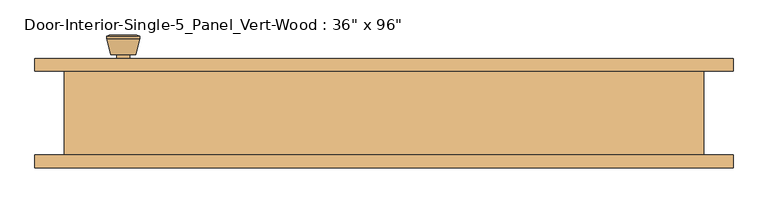
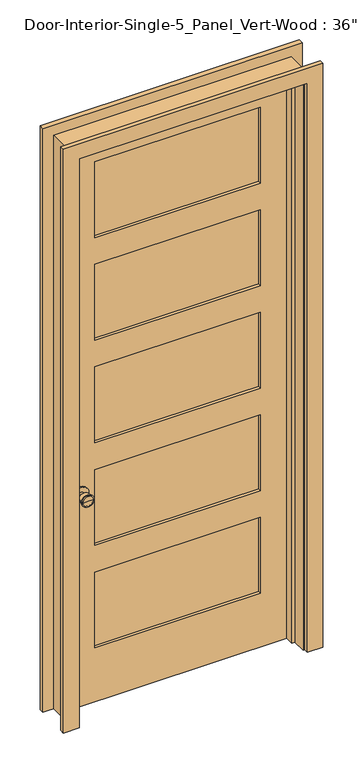
"""IFC4 building model written with IfcOpenShell, lengths in millimetres: door geometry."""

from ifc_helpers import new_model, si_unit, point, frame, frame_2d, origin, place, context, project, spatial, polyline, circle_curve, trimmed, segment, composite_curve, outline, extrude, faceted_brep, source, transform, mapped, element, save
from ifc_brep_helpers import plane_surface, cylinder_surface, revolved_surface, advanced_brep


def door_7b78131b(model_context):
    return source(origin(), model_context, "Body", "SolidModel", [
        advanced_brep(
        [(-393.7, 19.4, 914.4), (-383.7, 19.4, 914.4), (-403.7, 19.4, 914.4), (-373.2241324, -29.6, 914.4), (-393.7, -29.6, 914.4), (-414.1758676, -29.6, 914.4), (-368.7, -27.7721319, 914.4), (-418.7, -27.7721319, 914.4), (-368.7, -24.3084537, 914.4), (-418.7, -24.3084537, 914.4), (-375.063764, 0.4, 914.4), (-412.336236, 0.4, 914.4), (-383.7, 0.4, 914.4), (-403.7, 0.4, 914.4)],
        [
            (0, 1),
            (1, 2, circle_curve(frame((-393.7, 19.4, 914.4), z_axis=(0.0, 1.0, 0.0), x_axis=(-1.0, 0.0, 0.0)), 10.0)),
            (2, 0),
            (2, 1, circle_curve(frame((-393.7, 19.4, 914.4), z_axis=(0.0, 1.0, 0.0), x_axis=(-1.0, 0.0, 0.0)), 10.0)),
            (3, 4),
            (4, 5),
            (5, 3, circle_curve(frame((-393.7, -29.6, 914.4), z_axis=(0.0, -1.0, 0.0), x_axis=(-1.0, 0.0, 0.0)), 20.4758676)),
            (3, 5, circle_curve(frame((-393.7, -29.6, 914.4), z_axis=(0.0, -1.0, 0.0), x_axis=(-1.0, 0.0, 0.0)), 20.4758676)),
            (6, 3),
            (5, 7),
            (7, 6, circle_curve(frame((-393.7, -27.7721319, 914.4), z_axis=(0.0, -1.0, 0.0), x_axis=(-1.0, 0.0, 0.0)), 25.0)),
            (6, 7, circle_curve(frame((-393.7, -27.7721319, 914.4), z_axis=(0.0, -1.0, 0.0), x_axis=(-1.0, 0.0, 0.0)), 25.0)),
            (8, 6),
            (7, 9),
            (9, 8, circle_curve(frame((-393.7, -24.3084537, 914.4), z_axis=(0.0, -1.0, 0.0), x_axis=(-1.0, 0.0, 0.0)), 25.0)),
            (8, 9, circle_curve(frame((-393.7, -24.3084537, 914.4), z_axis=(0.0, -1.0, 0.0), x_axis=(-1.0, 0.0, 0.0)), 25.0)),
            (10, 8),
            (9, 11),
            (11, 10, circle_curve(frame((-393.7, 0.4, 914.4), z_axis=(0.0, -1.0, 0.0), x_axis=(-1.0, 0.0, 0.0)), 18.636236)),
            (10, 11, circle_curve(frame((-393.7, 0.4, 914.4), z_axis=(0.0, -1.0, 0.0), x_axis=(-1.0, 0.0, 0.0)), 18.636236)),
            (12, 10),
            (11, 13),
            (13, 12, circle_curve(frame((-393.7, 0.4, 914.4), z_axis=(0.0, -1.0, 0.0), x_axis=(-1.0, 0.0, 0.0)), 10.0)),
            (12, 13, circle_curve(frame((-393.7, 0.4, 914.4), z_axis=(0.0, -1.0, 0.0), x_axis=(-1.0, 0.0, 0.0)), 10.0)),
            (1, 12),
            (13, 2),
        ],
        [
            plane_surface(frame((-393.7, 19.4, 914.4), z_axis=(0.0, 1.0, 0.0), x_axis=(-1.0, 0.0, 0.0))),
            plane_surface(frame((-393.7, -29.6, 914.4), z_axis=(0.0, -1.0, 0.0), x_axis=(-1.0, 0.0, 0.0))),
            revolved_surface(polyline([(-414.1758676, -29.6, 914.4), (-418.7, -27.7721319, 914.4)]), (-393.7, 19.4, 914.4), (0.0, 1.0, 0.0)),
            cylinder_surface(frame((-393.7, 19.4, 914.4), z_axis=(0.0, 1.0, 0.0), x_axis=(-1.0, 0.0, 0.0)), 25.0),
            revolved_surface(polyline([(-418.7, -24.3084537, 914.4), (-412.336236, 0.4, 914.4)]), (-393.7, 19.4, 914.4), (0.0, 1.0, 0.0)),
            plane_surface(frame((-393.7, 0.4, 914.4), z_axis=(0.0, 1.0, 0.0), x_axis=(-1.0, 0.0, 0.0))),
            cylinder_surface(frame((-393.7, 19.4, 914.4), z_axis=(0.0, 1.0, 0.0), x_axis=(-1.0, 0.0, 0.0)), 10.0),
        ],
        [
            (0, [[1, 2, 3]]),
            (0, [[-3, 4, -1]]),
            (1, [[5, 6, 7]]),
            (1, [[-6, -5, 8]]),
            (2, [[9, -7, 10, 11]]),
            (2, [[-10, -8, -9, 12]]),
            (3, [[13, -11, 14, 15]]),
            (3, [[-14, -12, -13, 16]]),
            (4, [[17, -15, 18, 19]]),
            (4, [[-18, -16, -17, 20]]),
            (5, [[21, -19, 22, 23]]),
            (5, [[-22, -20, -21, 24]]),
            (6, [[25, -23, 26, -2]]),
            (6, [[-26, -24, -25, -4]]),
        ],
    ),
        extrude(outline(composite_curve([segment(trimmed(circle_curve(frame_2d((914.4, -393.7)), 30.0), [point((914.4, -423.7))], [point((914.4, -363.7))], False, "CARTESIAN"), True, "CONTINUOUS"), segment(trimmed(circle_curve(frame_2d((914.4, -393.7)), 30.0), [point((914.4, -363.7))], [point((914.4, -423.7))], False, "CARTESIAN"), True, "CONTINUOUS")], self_intersect=False)), frame((0.0, 19.4, 0.0), z_axis=(0.0, 1.0, 0.0), x_axis=(0.0, 0.0, 1.0)), (0.0, 0.0, 1.0), 6.0),
        advanced_brep(
        [(-393.7, 66.325, 914.4), (-403.7, 66.325, 914.4), (-383.7, 66.325, 914.4), (-373.2241324, 115.325, 914.4), (-414.1758676, 115.325, 914.4), (-393.7, 115.325, 914.4), (-368.7, 113.4971319, 914.4), (-418.7, 113.4971319, 914.4), (-368.7, 110.0334537, 914.4), (-418.7, 110.0334537, 914.4), (-375.063764, 85.325, 914.4), (-412.336236, 85.325, 914.4), (-383.7, 85.325, 914.4), (-403.7, 85.325, 914.4)],
        [
            (0, 1),
            (1, 2, circle_curve(frame((-393.7, 66.325, 914.4), z_axis=(0.0, -1.0, 0.0), x_axis=(-1.0, 0.0, 0.0)), 10.0)),
            (2, 0),
            (2, 1, circle_curve(frame((-393.7, 66.325, 914.4), z_axis=(0.0, -1.0, 0.0), x_axis=(-1.0, 0.0, 0.0)), 10.0)),
            (3, 4, circle_curve(frame((-393.7, 115.325, 914.4), z_axis=(0.0, 1.0, 0.0), x_axis=(-1.0, 0.0, 0.0)), 20.4758676)),
            (4, 5),
            (5, 3),
            (4, 3, circle_curve(frame((-393.7, 115.325, 914.4), z_axis=(0.0, 1.0, 0.0), x_axis=(-1.0, 0.0, 0.0)), 20.4758676)),
            (6, 7, circle_curve(frame((-393.7, 113.4971319, 914.4), z_axis=(0.0, 1.0, 0.0), x_axis=(-1.0, 0.0, 0.0)), 25.0)),
            (7, 4),
            (3, 6),
            (7, 6, circle_curve(frame((-393.7, 113.4971319, 914.4), z_axis=(0.0, 1.0, 0.0), x_axis=(-1.0, 0.0, 0.0)), 25.0)),
            (8, 9, circle_curve(frame((-393.7, 110.0334537, 914.4), z_axis=(0.0, 1.0, 0.0), x_axis=(-1.0, 0.0, 0.0)), 25.0)),
            (9, 7),
            (6, 8),
            (9, 8, circle_curve(frame((-393.7, 110.0334537, 914.4), z_axis=(0.0, 1.0, 0.0), x_axis=(-1.0, 0.0, 0.0)), 25.0)),
            (10, 11, circle_curve(frame((-393.7, 85.325, 914.4), z_axis=(0.0, 1.0, 0.0), x_axis=(-1.0, 0.0, 0.0)), 18.636236)),
            (11, 9),
            (8, 10),
            (11, 10, circle_curve(frame((-393.7, 85.325, 914.4), z_axis=(0.0, 1.0, 0.0), x_axis=(-1.0, 0.0, 0.0)), 18.636236)),
            (12, 13, circle_curve(frame((-393.7, 85.325, 914.4), z_axis=(0.0, 1.0, 0.0), x_axis=(-1.0, 0.0, 0.0)), 10.0)),
            (13, 11),
            (10, 12),
            (13, 12, circle_curve(frame((-393.7, 85.325, 914.4), z_axis=(0.0, 1.0, 0.0), x_axis=(-1.0, 0.0, 0.0)), 10.0)),
            (1, 13),
            (12, 2),
        ],
        [
            plane_surface(frame((-393.7, 66.325, 914.4), z_axis=(0.0, -1.0, 0.0), x_axis=(-1.0, 0.0, 0.0))),
            plane_surface(frame((-393.7, 115.325, 914.4), z_axis=(0.0, 1.0, 0.0), x_axis=(-1.0, 0.0, 0.0))),
            revolved_surface(polyline([(-414.1758676, 115.325, 914.4), (-418.7, 113.4971319, 914.4)]), (-393.7, 66.325, 914.4), (0.0, -1.0, 0.0)),
            cylinder_surface(frame((-393.7, 66.325, 914.4), z_axis=(0.0, -1.0, 0.0), x_axis=(-1.0, 0.0, 0.0)), 25.0),
            revolved_surface(polyline([(-418.7, 110.0334537, 914.4), (-412.336236, 85.325, 914.4)]), (-393.7, 66.325, 914.4), (0.0, -1.0, 0.0)),
            plane_surface(frame((-393.7, 85.325, 914.4), z_axis=(0.0, -1.0, 0.0), x_axis=(-1.0, 0.0, 0.0))),
            cylinder_surface(frame((-393.7, 66.325, 914.4), z_axis=(0.0, -1.0, 0.0), x_axis=(-1.0, 0.0, 0.0)), 10.0),
        ],
        [
            (0, [[1, 2, 3]]),
            (0, [[-3, 4, -1]]),
            (1, [[5, 6, 7]]),
            (1, [[8, -7, -6]]),
            (2, [[9, 10, -5, 11]]),
            (2, [[12, -11, -8, -10]]),
            (3, [[13, 14, -9, 15]]),
            (3, [[16, -15, -12, -14]]),
            (4, [[17, 18, -13, 19]]),
            (4, [[20, -19, -16, -18]]),
            (5, [[21, 22, -17, 23]]),
            (5, [[24, -23, -20, -22]]),
            (6, [[-2, 25, -21, 26]]),
            (6, [[-4, -26, -24, -25]]),
        ],
    ),
        extrude(outline(composite_curve([segment(trimmed(circle_curve(frame_2d((914.4, -393.7)), 30.0), [point((914.4, -423.7))], [point((914.4, -363.7))], False, "CARTESIAN"), True, "CONTINUOUS"), segment(trimmed(circle_curve(frame_2d((914.4, -393.7)), 30.0), [point((914.4, -363.7))], [point((914.4, -423.7))], False, "CARTESIAN"), True, "CONTINUOUS")], self_intersect=False)), frame((0.0, 60.325, 0.0), z_axis=(0.0, 1.0, 0.0), x_axis=(0.0, 0.0, 1.0)), (0.0, 0.0, 1.0), 6.0),
        faceted_brep([(482.6, 60.325, 0.0), (482.6, -66.675, 0.0), (457.2, -66.675, 0.0), (457.2, -9.525, 0.0), (444.5, -9.525, 0.0), (444.5, 25.4, 0.0), (457.2, 25.4, 0.0), (457.2, 60.325, 0.0), (482.6, 60.325, 2463.8), (482.6, -66.675, 2463.8), (-482.6, -66.675, 2463.8), (-482.6, -66.675, 0.0), (-457.2, -66.675, 0.0), (-457.2, -66.675, 2438.4), (457.2, -66.675, 2438.4), (457.2, -9.525, 2438.4), (-457.2, -9.525, 2438.4), (-457.2, -9.525, 0.0), (-444.5, -9.525, 0.0), (-444.5, -9.525, 2425.7), (444.5, -9.525, 2425.7), (444.5, 25.4, 2425.7), (-444.5, 25.4, 2425.7), (-444.5, 25.4, 0.0), (-457.2, 25.4, 0.0), (-457.2, 25.4, 2438.4), (457.2, 25.4, 2438.4), (457.2, 60.325, 2438.4), (-457.2, 60.325, 2438.4), (-457.2, 60.325, 0.0), (-482.6, 60.325, 0.0), (-482.6, 60.325, 2463.8)], [[[0, 1, 2, 3, 4, 5, 6, 7]], [[1, 0, 8, 9]], [[2, 1, 9, 10, 11, 12, 13, 14]], [[3, 2, 14, 15]], [[4, 3, 15, 16, 17, 18, 19, 20]], [[5, 4, 20, 21]], [[6, 5, 21, 22, 23, 24, 25, 26]], [[7, 6, 26, 27]], [[0, 7, 27, 28, 29, 30, 31, 8]], [[9, 8, 31, 10]], [[15, 14, 13, 16]], [[21, 20, 19, 22]], [[27, 26, 25, 28]], [[30, 29, 24, 23, 18, 17, 12, 11]], [[10, 31, 30, 11]], [[16, 13, 12, 17]], [[22, 19, 18, 23]], [[28, 25, 24, 29]]]),
        extrude(outline(polyline([(2438.4, -457.2), (0.0, -457.2), (0.0, 457.2), (2438.4, 457.2), (2438.4, -457.2)]), holes=[polyline([(2319.3375, -336.55), (2319.3375, 336.55), (1993.265, 336.55), (1993.265, -336.55), (2319.3375, -336.55)]), polyline([(557.8475, -336.55), (557.8475, 336.55), (231.775, 336.55), (231.775, -336.55), (557.8475, -336.55)]), polyline([(1438.5925, -336.55), (1438.5925, 336.55), (1112.52, 336.55), (1112.52, -336.55), (1438.5925, -336.55)]), polyline([(1878.965, -336.55), (1878.965, 336.55), (1552.8925, 336.55), (1552.8925, -336.55), (1878.965, -336.55)]), polyline([(998.22, -336.55), (998.22, 336.55), (672.1475, 336.55), (672.1475, -336.55), (998.22, -336.55)])]), frame((0.0, 25.4, 0.0), z_axis=(0.0, 1.0, 0.0), x_axis=(0.0, 0.0, 1.0)), (0.0, 0.0, 1.0), 34.925),
        extrude(outline(polyline([(336.55, 37.0416667), (-336.55, 37.0416667), (-336.55, 48.6833333), (336.55, 48.6833333), (336.55, 37.0416667)])), frame((0.0, 0.0, 1993.265), z_axis=(0.0, 0.0, 1.0), x_axis=(1.0, 0.0, 0.0)), (0.0, 0.0, 1.0), 326.0725),
        extrude(outline(polyline([(336.55, 37.0416667), (-336.55, 37.0416667), (-336.55, 48.6833333), (336.55, 48.6833333), (336.55, 37.0416667)])), frame((0.0, 0.0, 1552.8925), z_axis=(0.0, 0.0, 1.0), x_axis=(1.0, 0.0, 0.0)), (0.0, 0.0, 1.0), 326.0725),
        extrude(outline(polyline([(336.55, 37.0416667), (-336.55, 37.0416667), (-336.55, 48.6833333), (336.55, 48.6833333), (336.55, 37.0416667)])), frame((0.0, 0.0, 672.1475), z_axis=(0.0, 0.0, 1.0), x_axis=(1.0, 0.0, 0.0)), (0.0, 0.0, 1.0), 326.0725),
        extrude(outline(polyline([(336.55, 37.0416667), (-336.55, 37.0416667), (-336.55, 48.6833333), (336.55, 48.6833333), (336.55, 37.0416667)])), frame((0.0, 0.0, 231.775), z_axis=(0.0, 0.0, 1.0), x_axis=(1.0, 0.0, 0.0)), (0.0, 0.0, 1.0), 326.0725),
        extrude(outline(polyline([(336.55, 37.0416667), (-336.55, 37.0416667), (-336.55, 48.6833333), (336.55, 48.6833333), (336.55, 37.0416667)])), frame((0.0, 0.0, 1112.52), z_axis=(0.0, 0.0, 1.0), x_axis=(1.0, 0.0, 0.0)), (0.0, 0.0, 1.0), 326.0725),
        extrude(outline(polyline([(0.0, 463.55), (0.0, 527.05), (2508.25, 527.05), (2508.25, -527.05), (0.0, -527.05), (0.0, -463.55), (2444.75, -463.55), (2444.75, 463.55), (0.0, 463.55)])), frame((0.0, 60.325, 0.0), z_axis=(0.0, 1.0, 0.0), x_axis=(0.0, 0.0, 1.0)), (0.0, 0.0, 1.0), 19.05),
        extrude(outline(polyline([(0.0, 463.55), (0.0, 527.05), (2508.25, 527.05), (2508.25, -527.05), (0.0, -527.05), (0.0, -463.55), (2444.75, -463.55), (2444.75, 463.55), (0.0, 463.55)])), frame((0.0, -85.725, 0.0), z_axis=(0.0, 1.0, 0.0), x_axis=(0.0, 0.0, 1.0)), (0.0, 0.0, 1.0), 19.05),
    ])


if __name__ == "__main__":
    model = new_model("IFC4")
    model_context = context("Model", 3, world=origin())
    ifc_project = project(units=[si_unit("LENGTHUNIT", "METRE", prefix="MILLI")], contexts=[model_context])
    site = spatial("IfcSite", under=ifc_project)
    building = spatial("IfcBuilding", under=site)
    placement = place(None, origin())
    door_shape = door_7b78131b(model_context)
    element("IfcDoor", 1, ObjectType="Door-Interior-Single-5_Panel_Vert-Wood : 36\" x 96\"", at=placement, inside=building, context=model_context, shape_type="MappedRepresentation", body=[
        mapped(door_shape, transform((0.0, 0.0, 0.0), x_axis=(1.0, 0.0, 0.0), y_axis=(0.0, 1.0, 0.0), z_axis=(0.0, 0.0, 1.0))),
    ])
    save(model, "model.ifc")

# Revit data of these elements
# Type "Door-Interior-Single-5_Panel_Vert-Wood : 36\" x 96\""
#   Type Mark = "8"
#   Assembly Code = "C1020300"
#   Analytic Construction = "Wooden"
#   Top Rail = 0' - 4 11/16"
#   Thickness = 0' - 1 3/8"
#   Thermal Resistance (R) = 2.5876 (h·ft²·°F)/BTU
#   Swing Angle [instance default] = 90.00°
#   Stiles = 0' - 4 3/4"
#   Rough Width = 3' - 2"
#   Rough Height = 8' - 1"
#   Intermediate Rail = 0' - 4 1/2"
#   Height = 8' - 0"
#   Width = 3' - 0"
#   Heat Transfer Coefficient (U) = 0.3865 BTU/(h·ft²·°F)
#   Bottom Rail = 0' - 9 1/8"
#   Trim Material = Cherry
#   Panel Material = Cherry
#   Frame Material = Cherry
#   Door Handle Material = Aluminum
#   Visual Light Transmittance = 0
#   Solar Heat Gain Coefficient = 0
#   Wall Closure = (empty or 0)
#   Function = (empty or 0)
# Element 1 (IfcDoor, "Door-Interior-Single-5_Panel_Vert-Wood : 36\" x 96\"")
#   Materials on its faces: "Cherry", "Aluminum"
# Materials
#   "Cherry": class "Wood", colour RGB 226 177 128, transparency 0, Description = "Prunus Serotina", Cost = 0
#   "Aluminum": class "Metal", colour RGB 247 247 247, transparency 0, Description = "Aluminum 6061", Cost = 0
